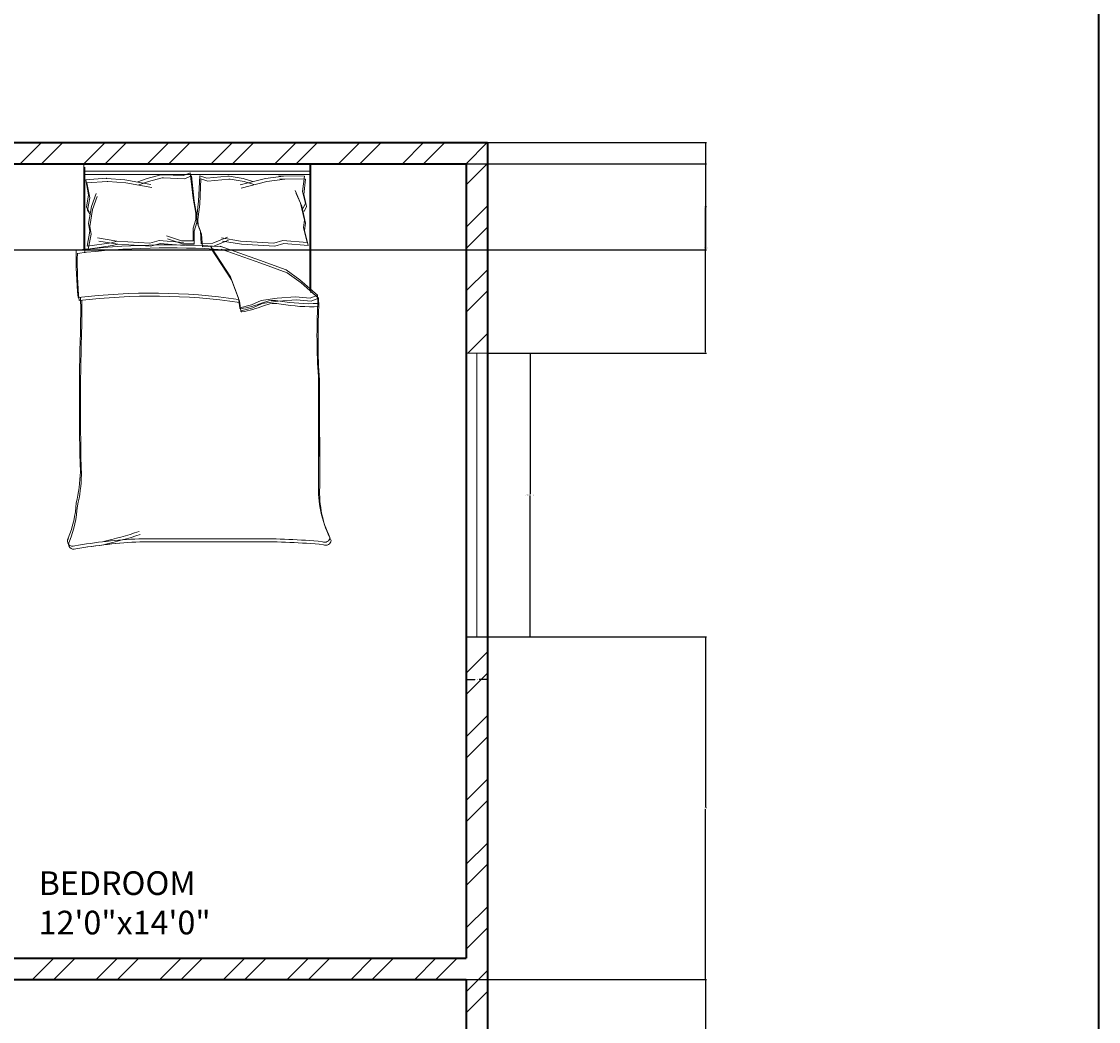
# Model space of a CAD drawing. Units: inches. Extents: x 392 to 1254, y 1207 to 2665.
# Tile 14 of 15: x 1026 to 1254, y 2043 to 2255. Entities that reach past the tile are written whole.
import ezdxf

# ---------------------------------------------------------------- set-up
doc = ezdxf.new("R2010")
doc.units = ezdxf.units.IN
for name, color, linetype, lineweight in [('A-ANNO-DIMS', 2, 'Continuous', 18), ('A-ANNO-TTLB', 7, 'Continuous', 35), ('A-AREA-IDEN', 7, 'Continuous', 18), ('A-FURN', 8, 'Continuous', 13), ('A-GLAZ', 4, 'Continuous', 18), ('A-WALL', 7, 'Continuous', 35), ('A-WALL-PATT', 252, 'Continuous', 13)]:
    doc.layers.add(name, color=color, linetype=linetype, lineweight=lineweight)
doc.styles.get("Standard").update_dxf_attribs({"font": 'arial.ttf'})
doc.dimstyles.get("Standard").update_dxf_attribs({"dimtxt": 0.18, "dimasz": 0.18, "dimexe": 0.18, "dimexo": 0.0625, "dimgap": 0.09, "dimtad": 0, "dimtih": 1, "dimtoh": 1, "dimdec": 4, "dimzin": 0, "dimdsep": 46, "dimtxsty": 'Standard', "dimcen": 0.09, "dimadec": 0, "dimazin": 0, "dimtfac": 1, "dimtdec": 4, "dimtofl": 0, "dimtmove": 0, "dimatfit": 3, "dimfxl": 1, "dimtolj": 1, "dimtzin": 0, "dimarcsym": 0})

# ---------------------------------------------------------------- blocks, each defined once
blk = doc.blocks.new('BED-DOUBLE')
for p, q in [((3.47, 63.33), (3.47, 81.44)), ((3.47, 79.91), (51.27, 79.91)), ((3.48, 63.33), (3.48, 81.44)), ((3.48, 79.91), (51.27, 79.91)), ((3.7, 62.69), (3.7, 80.8)), ((3.7, 62.69), (3.7, 80.8)), ((51.27, 81.44), (51.27, 54.83)), ((51.27, 81.44), (51.27, 54.83)), ((51.49, 81.44), (51.49, 80.8)), ((51.49, 80.8), (51.49, 54.19)), ((51.49, 80.8), (51.49, 54.19)), ((3.7, 79.27), (51.49, 79.27)), ((3.7, 79.27), (51.49, 79.27)), ((3.89, 78.13), (4.47, 74.95)), ((3.89, 78.13), (4.47, 74.95)), ((3.9, 78.1), (8.18, 78.43)), ((3.9, 78.1), (8.18, 78.43)), ((4.12, 77.49), (4.7, 74.31)), ((4.12, 77.49), (4.7, 74.31)), ((4.13, 77.47), (8.41, 77.79)), ((4.13, 77.47), (8.41, 77.79)), ((8.18, 78.43), (8.28, 78.42)), ((8.18, 78.43), (8.28, 78.42)), ((8.28, 78.42), (12.11, 78.13)), ((8.28, 78.42), (12.11, 78.13)), ((8.41, 77.79), (8.51, 77.78)), ((8.41, 77.79), (8.51, 77.78)), ((8.51, 77.78), (12.34, 77.49)), ((8.51, 77.78), (12.34, 77.49)), ((12.11, 78.13), (17.6, 77.11)), ((12.11, 78.13), (17.6, 77.11)), ((12.34, 77.49), (17.83, 76.48)), ((12.34, 77.49), (17.83, 76.48)), ((14.85, 77.69), (16.88, 78.42)), ((14.85, 77.69), (16.88, 78.42)), ((15.08, 77.05), (17.11, 77.78)), ((15.08, 77.05), (17.11, 77.78)), ((16.88, 78.42), (19.77, 79.14)), ((16.88, 78.42), (19.77, 79.14)), ((17.11, 77.78), (20, 78.5)), ((17.11, 77.78), (20, 78.5)), ((19.77, 79.14), (20.09, 79.14)), ((19.77, 79.14), (20.09, 79.14)), ((20, 78.5), (20.32, 78.5)), ((20, 78.5), (20.32, 78.5)), ((20.09, 79.14), (24.54, 78.99)), ((20.09, 79.14), (24.54, 78.99)), ((20.32, 78.5), (24.77, 78.35)), ((20.32, 78.5), (24.77, 78.35)), ((24.54, 78.99), (25.98, 79.57)), ((24.54, 78.99), (25.98, 79.57)), ((24.77, 78.35), (26.21, 78.93)), ((24.77, 78.35), (26.21, 78.93)), ((25.98, 79.57), (26.56, 74.22)), ((25.98, 79.57), (26.56, 74.22)), ((26.21, 78.93), (26.79, 73.58)), ((26.21, 78.93), (26.79, 73.58)), ((27.98, 78.95), (27.73, 73.58)), ((27.98, 78.95), (27.73, 73.58)), ((28.21, 78.31), (27.96, 72.94)), ((28.21, 78.31), (27.96, 72.94)), ((29.46, 78.46), (27.98, 78.95)), ((29.46, 78.46), (27.98, 78.95)), ((29.68, 77.82), (28.21, 78.31)), ((29.68, 77.82), (28.21, 78.31)), ((33.88, 78.89), (29.46, 78.46)), ((33.88, 78.89), (29.46, 78.46)), ((34.11, 78.25), (29.68, 77.82)), ((34.11, 78.25), (29.68, 77.82)), ((34.2, 78.91), (33.88, 78.89)), ((34.2, 78.91), (33.88, 78.89)), ((34.43, 78.27), (34.11, 78.25)), ((34.43, 78.27), (34.11, 78.25)), ((37.14, 78.36), (34.2, 78.91)), ((37.14, 78.36), (34.2, 78.91)), ((37.36, 77.73), (34.43, 78.27)), ((37.36, 77.73), (34.43, 78.27)), ((41.91, 78.37), (36.49, 77.02)), ((41.91, 78.37), (36.5, 77.02)), ((42.14, 77.73), (36.72, 76.38)), ((42.14, 77.73), (36.72, 76.38)), ((39.2, 77.77), (37.14, 78.36)), ((39.2, 77.77), (37.14, 78.36)), ((39.43, 77.13), (37.36, 77.73)), ((39.43, 77.13), (37.36, 77.73)), ((45.71, 78.9), (41.91, 78.37)), ((45.71, 78.9), (41.91, 78.37)), ((45.94, 78.26), (42.14, 77.73)), ((45.94, 78.26), (42.14, 77.73)), ((50.11, 78.89), (44.71, 78.98)), ((44.71, 78.98), (45.71, 78.9)), ((50.11, 78.89), (44.71, 78.98)), ((44.71, 78.98), (45.71, 78.9)), ((50.34, 78.25), (44.94, 78.34)), ((44.94, 78.34), (45.94, 78.26)), ((50.34, 78.25), (44.94, 78.34)), ((44.94, 78.34), (45.94, 78.26)), ((50.11, 78.89), (49.73, 75.67)), ((50.11, 78.89), (49.73, 75.67)), ((50.34, 78.25), (49.96, 75.04)), ((50.34, 78.25), (49.96, 75.04)), ((5.05, 72.49), (6.06, 75.23)), ((5.05, 72.49), (6.06, 75.23)), ((49.31, 73.19), (48.13, 75.86)), ((49.31, 73.19), (48.13, 75.86)), ((49.54, 72.55), (48.36, 75.22)), ((49.54, 72.55), (48.36, 75.22)), ((49.73, 75.67), (50.33, 73.1)), ((49.73, 75.67), (50.33, 73.1)), ((4.47, 74.95), (4.04, 72.34)), ((4.47, 74.95), (4.04, 72.34)), ((4.7, 74.31), (4.27, 71.7)), ((4.7, 74.31), (4.27, 71.7)), ((5.28, 71.85), (6.29, 74.6)), ((5.28, 71.85), (6.29, 74.6)), ((26.56, 74.22), (27.14, 71.04)), ((26.56, 74.22), (27.14, 71.04)), ((26.79, 73.58), (27.37, 70.4)), ((26.79, 73.58), (27.37, 70.4)), ((27.73, 73.58), (27.35, 70.36)), ((27.73, 73.58), (27.35, 70.36)), ((27.96, 72.94), (27.58, 69.73)), ((27.96, 72.94), (27.58, 69.73)), ((50.11, 69.61), (49.31, 73.19)), ((50.11, 69.61), (49.31, 73.19)), ((50.33, 73.1), (49.81, 72.06)), ((50.33, 73.1), (49.81, 72.06)), ((49.96, 75.04), (50.56, 72.47)), ((49.96, 75.04), (50.56, 72.47)), ((4.04, 72.34), (4.62, 71.33)), ((4.04, 72.34), (4.62, 71.33)), ((4.27, 71.7), (4.85, 70.69)), ((4.27, 71.7), (4.85, 70.69)), ((4.47, 68.87), (5.05, 72.49)), ((4.47, 68.87), (5.05, 72.49)), ((4.7, 68.23), (5.28, 71.85)), ((4.7, 68.23), (5.28, 71.85)), ((27.14, 71.04), (27.14, 69.74)), ((27.14, 71.04), (27.14, 69.74)), ((50.34, 68.97), (49.54, 72.55)), ((50.34, 68.97), (49.54, 72.55)), ((50.56, 72.47), (50.04, 71.42)), ((50.56, 72.47), (50.04, 71.42)), ((4.76, 67.28), (4.47, 68.87)), ((4.76, 67.28), (4.47, 68.87)), ((27.14, 69.74), (26.56, 67.86)), ((27.14, 69.74), (26.56, 67.86)), ((27.37, 69.1), (26.79, 67.22)), ((27.37, 69.1), (26.79, 67.22)), ((27.35, 70.36), (27.44, 69.07)), ((27.35, 70.36), (27.44, 69.07)), ((27.37, 70.4), (27.37, 69.1)), ((27.37, 70.4), (27.37, 69.1)), ((27.44, 69.07), (28.13, 67.23)), ((27.44, 69.07), (28.13, 67.23)), ((27.58, 69.73), (27.66, 68.43)), ((27.58, 69.73), (27.66, 68.43)), ((27.66, 68.43), (28.36, 66.59)), ((27.66, 68.43), (28.36, 66.59)), ((49.92, 68.01), (50.11, 69.61)), ((49.92, 68.01), (50.11, 69.61)), ((50.15, 67.37), (50.34, 68.97)), ((50.15, 67.37), (50.34, 68.97)), ((4.18, 64.1), (4.76, 67.28)), ((4.18, 64.1), (4.76, 67.28)), ((4.41, 63.46), (4.99, 66.64)), ((4.41, 63.46), (4.99, 66.64)), ((4.99, 66.64), (4.7, 68.23)), ((4.99, 66.64), (4.7, 68.23)), ((24.1, 65.18), (20.96, 66.27)), ((24.1, 65.18), (20.96, 66.27)), ((26.56, 67.86), (26.56, 65.18)), ((26.56, 67.86), (26.56, 65.18)), ((26.79, 67.22), (26.79, 64.54)), ((26.79, 67.22), (26.79, 64.54)), ((28.13, 67.23), (28.3, 64.55)), ((28.13, 67.23), (28.3, 64.55)), ((28.36, 66.59), (28.53, 63.91)), ((28.36, 66.59), (28.53, 63.91)), ((50.7, 64.87), (49.92, 68.01)), ((50.7, 64.87), (49.92, 68.01)), ((50.93, 64.23), (50.15, 67.37)), ((50.93, 64.23), (50.15, 67.37)), ((9.28, 64.82), (4.18, 64.1)), ((9.28, 64.82), (4.18, 64.1)), ((9.51, 64.19), (4.41, 63.46)), ((9.51, 64.19), (4.41, 63.46)), ((6.38, 65.81), (10.41, 65.15)), ((6.38, 65.81), (10.41, 65.15)), ((6.61, 65.17), (10.64, 64.51)), ((6.61, 65.17), (10.64, 64.51)), ((10.41, 65.15), (9.28, 64.82)), ((10.41, 65.15), (9.28, 64.82)), ((10.64, 64.51), (9.51, 64.19)), ((10.64, 64.51), (9.51, 64.19)), ((10.41, 65.15), (17.42, 64.72)), ((10.41, 65.15), (17.42, 64.72)), ((10.64, 64.51), (17.65, 64.08)), ((10.64, 64.51), (17.65, 64.08)), ((17.42, 64.72), (19.38, 65.27)), ((17.42, 64.72), (19.38, 65.27)), ((17.65, 64.08), (19.61, 64.63)), ((17.65, 64.08), (19.61, 64.63)), ((19.38, 65.27), (24.52, 64.87)), ((19.38, 65.27), (24.52, 64.87)), ((19.61, 64.63), (24.74, 64.23)), ((19.61, 64.63), (24.74, 64.23)), ((24.33, 64.54), (21.19, 65.63)), ((24.33, 64.54), (21.19, 65.63)), ((26.56, 65.18), (24.1, 65.18)), ((26.56, 65.18), (24.1, 65.18)), ((26.79, 64.54), (24.33, 64.54)), ((26.79, 64.54), (24.33, 64.54)), ((28.3, 64.55), (30.75, 64.7)), ((28.3, 64.55), (30.75, 64.7)), ((28.53, 63.91), (30.98, 64.06)), ((28.53, 63.91), (30.98, 64.06)), ((30.26, 64.06), (34.45, 57.57)), ((30.26, 64.06), (34.45, 57.57)), ((30.75, 64.7), (33.82, 65.99)), ((30.75, 64.7), (33.82, 65.99)), ((30.98, 64.06), (34.05, 65.35)), ((30.98, 64.06), (34.05, 65.35)), ((40.64, 61.13), (32.31, 64.06)), ((40.64, 61.13), (32.31, 64.06)), ((32.56, 65.81), (36.6, 65.15)), ((32.56, 65.81), (36.6, 65.15)), ((32.79, 65.17), (36.82, 64.51)), ((32.79, 65.17), (36.82, 64.51)), ((36.6, 65.15), (43.61, 64.72)), ((36.6, 65.15), (43.61, 64.72)), ((36.82, 64.51), (43.83, 64.08)), ((36.82, 64.51), (43.83, 64.08)), ((43.61, 64.72), (45.57, 65.27)), ((43.61, 64.72), (45.57, 65.27)), ((43.83, 64.08), (45.79, 64.63)), ((43.83, 64.08), (45.79, 64.63)), ((45.57, 65.27), (50.7, 64.87)), ((45.57, 65.27), (50.7, 64.87)), ((45.79, 64.63), (50.93, 64.23)), ((45.79, 64.63), (50.93, 64.23)), ((30.49, 63.42), (34.68, 56.93)), ((30.49, 63.42), (34.68, 56.93)), ((40.87, 60.49), (32.53, 63.42)), ((40.87, 60.49), (32.53, 63.42)), ((46.22, 59.11), (40.64, 61.13)), ((46.22, 59.11), (40.64, 61.13)), ((46.45, 58.47), (40.87, 60.49)), ((46.45, 58.47), (40.87, 60.49)), ((34.45, 57.57), (36.15, 53.08)), ((34.45, 57.57), (36.15, 53.08)), ((49.16, 56.95), (46.22, 59.11)), ((49.16, 56.95), (46.22, 59.11)), ((49.39, 56.31), (46.45, 58.47)), ((49.39, 56.31), (46.45, 58.47)), ((52.87, 53.7), (49.16, 56.95)), ((52.87, 53.7), (49.16, 56.95)), ((34.68, 56.93), (36.38, 52.44)), ((34.68, 56.93), (36.38, 52.44)), ((53.1, 53.06), (49.39, 56.31)), ((53.1, 53.06), (49.39, 56.31)), ((36.15, 53.08), (36.46, 51.07)), ((36.15, 53.08), (36.46, 51.07)), ((36.38, 52.44), (36.69, 50.43)), ((36.38, 52.44), (36.69, 50.43)), ((38.94, 51.68), (40.95, 52.61)), ((38.94, 51.68), (40.95, 52.61)), ((40.95, 52.61), (44.36, 53.08)), ((40.95, 52.61), (44.36, 53.08)), ((41.18, 51.97), (44.59, 52.44)), ((41.18, 51.97), (44.59, 52.44)), ((44.36, 53.08), (48.23, 53.39)), ((44.36, 53.08), (48.23, 53.39)), ((44.59, 52.44), (48.46, 52.75)), ((44.59, 52.44), (48.46, 52.75)), ((48.23, 53.39), (51.33, 53.08)), ((48.23, 53.39), (51.33, 53.08)), ((48.46, 52.75), (51.56, 52.44)), ((48.46, 52.75), (51.56, 52.44)), ((51.33, 53.08), (52.87, 53.7)), ((51.33, 53.08), (52.87, 53.7)), ((51.56, 52.44), (53.1, 53.06)), ((51.56, 52.44), (53.1, 53.06)), ((52.95, 51.95), (52.87, 53.7, 3.87)), ((52.95, 51.95), (52.87, 53.7, 3.87)), ((53.18, 51.31), (53.1, 53.06, 3.87)), ((53.18, 51.31), (53.1, 53.06, 3.87)), ((36.46, 51.07), (38.94, 51.68)), ((36.46, 51.07), (38.94, 51.68)), ((36.69, 50.43), (39.17, 51.05)), ((36.69, 50.43), (39.17, 51.05)), ((39.17, 51.05), (41.18, 51.97)), ((39.17, 51.05), (41.18, 51.97)), ((15.06, 2.2), (39.68, 2.2)), ((15.06, 2.2), (39.68, 2.2)), ((15.29, 1.56), (39.91, 1.56)), ((15.29, 1.56), (39.91, 1.56))]:
    blk.add_line(p, q)
for centre, radius, start, end in [((21.36, -100.61), 164.97, 86.0865, 96.7821), ((21.36, -100.61), 164.97, 86.0865, 96.7821), ((85.16, 61.35), 83.31, 178.7218, 185.604), ((85.16, 61.35), 83.31, 178.7218, 185.604), ((85.39, 60.71), 83.31, 178.7218, 185.604), ((85.39, 60.71), 83.31, 178.7218, 185.604), ((21.59, -101.25), 164.97, 86.0865, 96.7821), ((21.59, -101.25), 164.97, 86.0865, 96.7821), ((17.76, -74.87), 129.02, 81.7845, 96.9006), ((17.76, -74.87), 129.02, 81.7845, 96.9006), ((17.98, -75.51), 129.02, 81.7845, 96.9006), ((17.98, -75.51), 129.02, 81.7845, 96.9006), ((-167.31, 50.27), 170.11, 358.4762, 1.0082), ((-167.31, 50.27), 170.11, 358.4762, 1.0082), ((-167.08, 49.63), 170.11, 358.4762, 1.0082), ((-167.08, 49.63), 170.11, 358.4762, 1.0082), ((43.74, 46.38), 6.22, 78.6608, 113.7384), ((43.74, 46.38), 6.22, 78.6608, 113.7384), ((51.33, 88.1), 36.18, 259.8763, 272.5657), ((51.33, 88.1), 36.18, 259.8763, 272.5657), ((36.64, 51), 0.185, 160.2464, 271.1377), ((36.64, 51), 0.185, 160.2464, 271.1377), ((31.15, 79.96), 29.65, 280.6617, 289.8806), ((31.15, 79.96), 29.65, 280.6617, 289.8806), ((36.86, 50.36), 0.185, 160.2464, 271.1377), ((36.86, 50.36), 0.185, 160.2464, 271.1377), ((31.38, 79.32), 29.65, 280.6617, 289.8806), ((31.38, 79.32), 29.65, 280.6617, 289.8806), ((43.97, 45.74), 6.22, 78.6608, 113.7384), ((43.97, 45.74), 6.22, 78.6608, 113.7384), ((51.56, 87.46), 36.18, 259.8763, 272.5657), ((51.56, 87.46), 36.18, 259.8763, 272.5657), ((182.27, 45.13), 129.5, 176.9791, 183.8365), ((182.27, 45.13), 129.5, 176.9791, 183.8365), ((182.49, 44.49), 129.5, 176.9791, 183.8365), ((182.49, 44.49), 129.5, 176.9791, 183.8365), ((484.82, 30.83), 482.31, 178.2277, 181.7185), ((484.82, 30.83), 482.31, 178.2277, 181.7185), ((485.05, 30.19), 482.31, 178.2277, 181.7185), ((485.05, 30.19), 482.31, 178.2277, 181.7185), ((-4508.74, 13.62), 4561.86, 0.00217, 0.28689), ((-4508.74, 13.62), 4561.86, 0.00217, 0.28689), ((-4508.51, 12.98), 4561.86, 0.00217, 0.28689), ((-4508.52, 12.98), 4561.86, 0.00217, 0.28689), ((-26.9, 16.93), 29.63, 346.0648, 358.9113), ((-26.9, 16.93), 29.63, 346.0648, 358.9113), ((-26.67, 16.29), 29.63, 346.0648, 358.9113), ((-26.67, 16.29), 29.63, 346.0648, 358.9113), ((76.16, 12.78), 23.07, 177.4714, 206.4681), ((76.16, 12.78), 23.07, 177.4714, 206.4681), ((76.39, 12.14), 23.07, 177.4714, 206.4681), ((76.39, 12.14), 23.07, 177.4714, 206.4681), ((-21.66, 11.17), 23.56, 337.9751, 356.652), ((-21.66, 11.17), 23.56, 337.9751, 356.652), ((-21.43, 10.53), 23.56, 337.9751, 356.652), ((-21.43, 10.53), 23.56, 337.9751, 356.652), ((1.09, 1.72), 1.09, 146.1736, 293.4781), ((1.09, 1.72), 1.09, 146.1736, 293.4781), ((-17.22, 105.15), 106.46, 283.3832, 287.7053), ((-17.22, 105.15), 106.46, 283.3832, 287.7053), ((-16.99, 104.52), 106.46, 283.3832, 287.7053), ((-16.99, 104.52), 106.46, 283.3832, 287.7053), ((54.41, 2.57), 1.1, 242.6588, 356.02), ((54.41, 2.57), 1.1, 242.6588, 356.02), ((1.32, 1.09), 1.09, 146.1736, 293.4781), ((1.32, 1.09), 1.09, 146.1736, 293.4781), ((21.43, -119.39), 121.76, 92.9958, 99.4091), ((21.43, -119.39), 121.76, 92.9958, 99.4091), ((21.66, -120.03), 121.76, 92.9958, 99.4091), ((21.65, -120.03), 121.76, 92.9958, 99.4091), ((41.15, -130.83), 133.04, 84.4998, 90.6351), ((41.15, -130.83), 133.04, 84.4998, 90.6351), ((41.38, -131.47), 133.04, 84.4998, 90.6351), ((41.38, -131.47), 133.04, 84.4998, 90.6351), ((54.64, 1.93), 1.1, 242.6588, 356.02), ((54.64, 1.93), 1.1, 242.6588, 356.02)]:
    blk.add_arc(centre, radius, start, end)
blk = doc.blocks.new('WIN-60-A')
for p, q in [((0, 60), (4.5, 60)), ((4.5, 60), (2.25, 60)), ((2.25, 60), (2.25, 0)), ((2.25, 0), (0, 0)), ((0, 0), (4.5, 0))]:
    blk.add_line(p, q)
blk = doc.blocks.new('*D11')
at = {"layer": 'A-ANNO-DIMS', "color": 0, "lineweight": -2, "transparency": 16777216}
for p, q in [((1124.84, 2184.76), (1133.96, 2184.76)), ((1133.78, 2184.58), (1133.78, 2154.94)), ((1133.78, 2124.94), (1133.78, 2154.58)), ((1124.84, 2124.76), (1133.96, 2124.76))]:
    blk.add_line(p, q, dxfattribs=at)
at = {"layer": 'A-ANNO-DIMS', "color": 0, "transparency": 16777216}
for points in [[(1133.75, 2184.58), (1133.81, 2184.58), (1133.78, 2184.76)], [(1133.75, 2124.94), (1133.81, 2124.94), (1133.78, 2124.76)]]:
    blk.add_solid(points, dxfattribs=at)
at = {"layer": 'Defpoints', "color": 0, "transparency": 16777216}
for p in [(1124.78, 2184.76), (1124.78, 2124.76), (1133.78, 2124.76)]:
    blk.add_point(p, dxfattribs=at)
at = {"layer": 'A-ANNO-DIMS', "color": 0, "transparency": 16777216, "insert": (1133.78, 2154.76), "char_height": 0.18, "attachment_point": 5}
blk.add_mtext('\\A1;WINDOW A 60 TYP.', dxfattribs=at)
blk = doc.blocks.new('*D12')
at = {"layer": 'A-ANNO-DIMS', "color": 0, "lineweight": -2, "transparency": 16777216}
for p, q in [((1120.28, 2124.7), (1120.28, 2115.58)), ((1124.78, 2124.7), (1124.78, 2115.58)), ((1120.46, 2115.76), (1122.07, 2115.76)), ((1124.6, 2115.76), (1122.99, 2115.76))]:
    blk.add_line(p, q, dxfattribs=at)
at = {"layer": 'A-ANNO-DIMS', "color": 0, "transparency": 16777216}
for points in [[(1120.46, 2115.79), (1120.46, 2115.73), (1120.28, 2115.76)], [(1124.6, 2115.79), (1124.6, 2115.73), (1124.78, 2115.76)]]:
    blk.add_solid(points, dxfattribs=at)
at = {"layer": 'Defpoints', "color": 0, "transparency": 16777216}
for p in [(1120.28, 2124.76), (1124.78, 2124.76), (1120.28, 2115.76)]:
    blk.add_point(p, dxfattribs=at)
at = {"layer": 'A-ANNO-DIMS', "color": 0, "transparency": 16777216, "insert": (1122.53, 2115.76), "char_height": 0.18, "attachment_point": 5}
blk.add_mtext('\\A1;5 TYP.', dxfattribs=at)
blk = doc.blocks.new('*D34')
at = {"layer": 'A-ANNO-DIMS', "color": 0, "lineweight": -2, "transparency": 16777216}
for p, q in [((1120.34, 2124.76), (1171.06, 2124.76)), ((1170.88, 2124.58), (1170.88, 2088.71)), ((1170.88, 2052.48), (1170.88, 2088.35)), ((1120.34, 2052.3), (1171.06, 2052.3))]:
    blk.add_line(p, q, dxfattribs=at)
at = {"layer": 'A-ANNO-DIMS', "color": 0, "transparency": 16777216}
for points in [[(1170.85, 2124.58), (1170.91, 2124.58), (1170.88, 2124.76)], [(1170.85, 2052.48), (1170.91, 2052.48), (1170.88, 2052.3)]]:
    blk.add_solid(points, dxfattribs=at)
at = {"layer": 'Defpoints', "color": 0, "transparency": 16777216}
for p in [(1120.28, 2124.76), (1170.88, 2124.76), (1120.28, 2052.3)]:
    blk.add_point(p, dxfattribs=at)
at = {"layer": 'A-ANNO-DIMS', "color": 0, "transparency": 16777216, "insert": (1170.88, 2088.53), "char_height": 0.18, "attachment_point": 5}
blk.add_mtext('\\A1;72.47', dxfattribs=at)
blk = doc.blocks.new('*D39')
at = {"layer": 'A-ANNO-DIMS', "color": 0, "lineweight": -2, "transparency": 16777216}
for p, q in [((1124.84, 2229.3), (1171.06, 2229.3)), ((1170.88, 2229.12), (1170.88, 2207.21)), ((1170.88, 2184.94), (1170.88, 2206.85)), ((1124.84, 2184.76), (1171.06, 2184.76))]:
    blk.add_line(p, q, dxfattribs=at)
at = {"layer": 'A-ANNO-DIMS', "color": 0, "transparency": 16777216}
for points in [[(1170.85, 2229.12), (1170.91, 2229.12), (1170.88, 2229.3)], [(1170.85, 2184.94), (1170.91, 2184.94), (1170.88, 2184.76)]]:
    blk.add_solid(points, dxfattribs=at)
at = {"layer": 'Defpoints', "color": 0, "transparency": 16777216}
for p in [(1124.78, 2229.3), (1124.78, 2184.76), (1170.88, 2184.76)]:
    blk.add_point(p, dxfattribs=at)
at = {"layer": 'A-ANNO-DIMS', "color": 0, "transparency": 16777216, "insert": (1170.88, 2207.03), "char_height": 0.18, "attachment_point": 5}
blk.add_mtext('\\A1;44.535', dxfattribs=at)
blk = doc.blocks.new('*D40')
at = {"layer": 'A-ANNO-DIMS', "color": 0, "lineweight": -2, "transparency": 16777216}
for p, q in [((1120.34, 2052.3), (1171.06, 2052.3)), ((1170.88, 2052.12), (1170.88, 2022.56)), ((1170.88, 1992.64), (1170.88, 2022.19)), ((1120.34, 1992.46), (1171.06, 1992.46))]:
    blk.add_line(p, q, dxfattribs=at)
at = {"layer": 'A-ANNO-DIMS', "color": 0, "transparency": 16777216}
for points in [[(1170.85, 2052.12), (1170.91, 2052.12), (1170.88, 2052.3)], [(1170.85, 1992.64), (1170.91, 1992.64), (1170.88, 1992.46)]]:
    blk.add_solid(points, dxfattribs=at)
at = {"layer": 'Defpoints', "color": 0, "transparency": 16777216}
for p in [(1120.28, 2052.3), (1120.28, 1992.46), (1170.88, 1992.46)]:
    blk.add_point(p, dxfattribs=at)
at = {"layer": 'A-ANNO-DIMS', "color": 0, "transparency": 16777216, "insert": (1170.88, 2022.38), "char_height": 0.18, "attachment_point": 5}
blk.add_mtext('\\A1;59.84', dxfattribs=at)
blk = doc.blocks.new('*D79')
at = {"layer": 'A-ANNO-DIMS', "color": 0, "lineweight": -2, "transparency": 16777216}
for p, q in [((830.84, 2224.8), (1171.06, 2224.8)), ((1170.88, 2224.62), (1170.88, 2215.87)), ((1170.88, 2206.76), (1170.88, 2215.5)), ((830.84, 2206.58), (1171.06, 2206.58))]:
    blk.add_line(p, q, dxfattribs=at)
at = {"layer": 'A-ANNO-DIMS', "color": 0, "transparency": 16777216}
for points in [[(1170.85, 2224.62), (1170.91, 2224.62), (1170.88, 2224.8)], [(1170.85, 2206.76), (1170.91, 2206.76), (1170.88, 2206.58)]]:
    blk.add_solid(points, dxfattribs=at)
at = {"layer": 'Defpoints', "color": 0, "transparency": 16777216}
for p in [(830.78, 2224.8), (1170.88, 2224.8), (830.78, 2206.58)]:
    blk.add_point(p, dxfattribs=at)
at = {"layer": 'A-ANNO-DIMS', "color": 0, "transparency": 16777216, "insert": (1170.88, 2215.69), "char_height": 0.18, "attachment_point": 5}
blk.add_mtext('\\A1;18.22', dxfattribs=at)

msp = doc.modelspace()

# ---------------------------------------------------------------- hatches: boundary and pattern name
at = {"layer": 'A-WALL-PATT'}
h = msp.add_hatch(dxfattribs=at)
h.set_pattern_fill('ANSI32', color=256)
h.paths.add_polyline_path([(579.5309, 2227.0453), (579.5309, 2229.2953), (541.2807, 2229.2953), (541.2807, 2182.3091), (545.7807, 2182.3091), (545.7807, 2224.7953), (579.5309, 2224.7953)])
h.paths.add_polyline_path([(655.4442, 2229.2953), (627.5309, 2229.2953), (627.5309, 2224.7953), (655.4442, 2224.7953), (655.4442, 2227.0453)])
h.paths.add_polyline_path([(703.0758, 2229.2953), (678.5257, 2229.2953), (678.5257, 2227.0453), (678.5257, 2224.7953), (689.7807, 2224.7953), (689.7807, 2158.6973), (694.2807, 2158.6973), (694.2807, 2224.7953), (703.0758, 2224.7953)])
h.paths.add_polyline_path([(768.5767, 2229.2953), (727.0758, 2229.2953), (727.0758, 2224.7953), (742.2807, 2224.7953), (742.2807, 2128.7953), (694.2807, 2128.7953), (694.2807, 2134.0554), (689.7807, 2134.0554), (689.7807, 2090.2854), (694.2807, 2090.2854), (694.2807, 2124.2953), (742.2807, 2124.2953), (742.2807, 2052.2953), (795.2124, 2052.2953), (795.2124, 2054.5453), (795.2124, 2056.7953), (746.7807, 2056.7953), (746.7807, 2224.7953), (768.5767, 2224.7953)])
h.paths.add_polyline_path([(867.5089, 2229.2953), (804.5767, 2229.2953), (804.5767, 2224.7953), (830.7807, 2224.7953), (830.7807, 2056.7953), (826.9066, 2056.7953), (826.9066, 2052.2953), (830.7807, 2052.2953), (830.7807, 1886.6777, -0.01766664), (830.8602, 1884.2953), (835.0818, 1884.2953, -0.04411348), (835.2807, 1889.9369), (835.2807, 2052.2953), (839.418, 2052.2953), (839.418, 2056.7953), (835.2807, 2056.7953), (835.2807, 2224.7953), (867.5089, 2224.7953)])
h.paths.add_polyline_path([(939.8604, 2229.2953), (903.5089, 2229.2953), (903.5089, 2227.0453), (903.5089, 2224.7953), (919.2807, 2224.7953), (919.2807, 2056.7953), (870.6499, 2056.7953), (870.6499, 2052.2953), (923.7807, 2052.2953), (923.7807, 2124.2953), (971.7807, 2124.2953), (971.7807, 2089.7112), (974.0307, 2089.7112), (976.2807, 2089.7112), (976.2807, 2133.56), (974.0307, 2133.56), (971.7807, 2133.56), (971.7807, 2128.7953), (923.7807, 2128.7953), (923.7807, 2224.7953), (939.8604, 2224.7953)])
h.paths.add_polyline_path([(1124.7807, 2229.2953), (1009.403, 2229.2953), (1009.403, 2224.7953), (1120.2807, 2224.7953), (1120.2807, 2184.7605), (1124.7807, 2184.7605)])
h.paths.add_polyline_path([(1124.7807, 2124.7605), (1120.2807, 2124.7605), (1120.2807, 2056.7953), (976.2807, 2056.7953), (976.2807, 2061.471), (971.7807, 2061.471), (971.7807, 2047.7483), (974.0307, 2047.7483), (976.2807, 2047.7483), (976.2807, 2052.2953), (1120.2807, 2052.2953), (1120.2807, 1992.457), (1124.7807, 1992.457)])
h.paths.add_polyline_path([(1124.7807, 1932.457), (1122.5307, 1932.457), (1120.2807, 1932.457), (1120.2807, 1884.2953), (976.2807, 1884.2953), (976.2807, 2019.9536), (971.7807, 2019.9536), (971.7807, 1884.2953), (869.0911, 1884.2953), (869.0911, 1879.7953), (971.7807, 1879.7953), (1013.7807, 1879.7953), (1013.7807, 1831.7953), (971.7807, 1831.7953), (971.7807, 1822.3831), (974.0307, 1822.3831), (976.2807, 1822.3831), (976.2807, 1827.2953), (1013.7807, 1827.2953), (1025.6191, 1827.2953), (1025.6191, 1829.5453), (1025.6191, 1831.7953), (1018.2807, 1831.7953), (1018.2807, 1879.7953), (1120.2807, 1879.7953), (1120.2807, 1866.9192), (1124.7807, 1866.9192)])
h.paths.add_polyline_path([(1124.7807, 1842.9192), (1122.5307, 1842.9192), (1120.2807, 1842.9192), (1120.2807, 1831.7953), (1050.2021, 1831.7953), (1050.2021, 1827.2953), (1120.2807, 1827.2953), (1120.2807, 1781.4559), (1124.7807, 1781.4559)])
h.paths.add_polyline_path([(976.2807, 1790.8718), (971.7807, 1790.8718), (971.7807, 1648.3339), (976.2807, 1648.3339), (976.2807, 1654.7953), (1120.2807, 1654.7953), (1120.2807, 1626.3807), (1124.7807, 1626.3807), (1124.7807, 1721.4559), (1120.2807, 1721.4559), (1120.2807, 1659.2953), (976.2807, 1659.2953)])
h.paths.add_polyline_path([(1124.7807, 1566.3807), (1120.2807, 1566.3807), (1120.2807, 1486.7953), (1101.07, 1486.7953), (1101.07, 1482.2953), (1124.7807, 1482.2953)])
h.paths.add_polyline_path([(1041.07, 1484.5453), (1041.07, 1486.7953), (1006.2807, 1486.7953), (1006.2807, 1484.5453), (1006.2807, 1482.2953), (1041.07, 1482.2953)])
h.paths.add_polyline_path([(976.2807, 1617.5497), (974.0307, 1617.5497), (971.7807, 1617.5497), (971.7807, 1599.2953), (965.8041, 1599.2953), (965.8041, 1594.7953), (971.7807, 1594.7953), (971.7807, 1486.7953), (954.1249, 1486.7953), (954.1249, 1482.2953), (981.5717, 1482.2953), (981.5717, 1484.5453), (981.5717, 1486.7953), (976.2807, 1486.7953)])
h.paths.add_polyline_path([(930.1249, 1486.7953), (887.7807, 1486.7953), (887.7807, 1594.7953), (941.9141, 1594.7953), (941.9141, 1597.0453), (941.9141, 1599.2953), (887.7807, 1599.2953), (887.7807, 1659.2953), (863.5916, 1659.2953), (863.5916, 1654.7953), (883.2807, 1654.7953), (883.2807, 1438.7953), (782.7807, 1438.7953), (782.7807, 1486.7953), (782.7807, 1654.7953), (800.1309, 1654.7953), (800.1309, 1657.0453), (800.1309, 1659.2953), (778.2807, 1659.2953), (778.2807, 1599.2953), (721.7333, 1599.2953), (721.7333, 1597.0453), (721.7333, 1594.7953), (778.2807, 1594.7953), (778.2807, 1486.7953), (729.598, 1486.7953), (729.598, 1482.2953), (753.2885, 1482.2953), (753.2885, 1410.2953), (922.9852, 1410.2953), (922.9852, 1482.2953), (930.1249, 1482.2953)])
h.paths.add_polyline_path([(918.4852, 1482.2953), (918.4852, 1414.7953), (757.7885, 1414.7953), (757.7885, 1482.2953), (778.2807, 1482.2953), (778.2807, 1434.2953), (782.7807, 1434.2953), (887.7807, 1434.2953), (887.7807, 1438.7953), (887.7807, 1482.2953)], flags=16)
h.paths.add_polyline_path([(694.2807, 1594.7953), (700.4169, 1594.7953), (700.4169, 1597.0453), (700.4169, 1599.2953), (694.2807, 1599.2953), (694.2807, 1617.7503), (692.0307, 1617.7503), (689.7807, 1617.7503), (689.7807, 1486.7953), (682.7672, 1486.7953), (682.7672, 1482.2953), (705.598, 1482.2953), (705.598, 1484.5453), (705.598, 1486.7953), (694.2807, 1486.7953)])
h.paths.add_polyline_path([(545.7807, 1654.7953), (689.7807, 1654.7953), (689.7807, 1649.7691), (694.2807, 1649.7691), (694.2807, 1789.3981), (692.0307, 1789.3981), (689.7807, 1789.3981), (689.7807, 1659.2953), (545.7807, 1659.2953), (545.7807, 1714.4681), (543.5307, 1714.4681), (541.2807, 1714.4681), (541.2807, 1482.2953), (567.0628, 1482.2953), (567.0628, 1484.5453), (567.0628, 1486.7953), (545.7807, 1486.7953)])
h.paths.add_polyline_path([(545.7807, 1827.2953), (620.2247, 1827.2953), (620.2247, 1829.5453), (620.2247, 1831.7953), (545.7807, 1831.7953), (545.7807, 1846.8518), (541.2807, 1846.8518), (541.2807, 1774.4681), (545.7807, 1774.4681)])
h.paths.add_polyline_path([(797.0944, 1884.2953), (694.2807, 1884.2953), (694.2807, 2019.0288), (692.0307, 2019.0288), (689.7807, 2019.0288), (689.7807, 1884.2953), (545.7807, 1884.2953), (545.7807, 1951.8244), (541.2807, 1951.8244), (541.2807, 1870.8518), (543.5307, 1870.8518), (545.7807, 1870.8518), (545.7807, 1879.7953), (647.7807, 1879.7953), (647.7807, 1831.7953), (642.6413, 1831.7953), (642.6413, 1827.2953), (652.2807, 1827.2953), (689.7807, 1827.2953), (689.7807, 1821.0531), (694.2807, 1821.0531), (694.2807, 1831.7953), (652.2807, 1831.7953), (652.2807, 1879.7953), (797.0944, 1879.7953), (797.0944, 1882.0453)])
h.paths.add_polyline_path([(545.7807, 2122.3091), (541.2807, 2122.3091), (541.2807, 2011.8244), (543.5307, 2011.8244), (545.7807, 2011.8244), (545.7807, 2052.2953), (689.7807, 2052.2953), (689.7807, 2048.2048), (694.2807, 2048.2048), (694.2807, 2061.3129), (692.0307, 2061.3129), (689.7807, 2061.3129), (689.7807, 2056.7953), (545.7807, 2056.7953)])

# ---------------------------------------------------------------- linework, layer by layer
at = {"layer": 'A-ANNO-TTLB'}
msp.add_lwpolyline([(391.939, 2664.8979), (1253.97, 2664.8979), (1253.97, 1207.2611), (391.939, 1207.2611)], close=True, dxfattribs=at)
at = {"layer": 'A-WALL'}
for p, q in [((1007.5313, 2229.2953), (1124.7807, 2229.2953)), ((1124.7807, 2229.2953), (1124.7807, 1482.2953)), ((1009.403, 2224.7953), (1120.2807, 2224.7953)), ((1120.2807, 2224.7953), (1120.2807, 2056.7953)), ((976.2807, 2056.7953), (1120.2807, 2056.7953)), ((976.2807, 2052.2953), (1120.2807, 2052.2953)), ((1120.2807, 2052.2953), (1120.2807, 1884.2953))]:
    msp.add_line(p, q, dxfattribs=at)

# ---------------------------------------------------------------- block references
at = {"layer": 'A-FURN'}
msp.add_blockref('BED-DOUBLE', (1035.9344, 2143.3004), dxfattribs=at)
at = {"layer": 'A-GLAZ', "rotation": 180}
msp.add_blockref('WIN-60-A', (1124.7804, 2184.7606), dxfattribs=at)

# ---------------------------------------------------------------- texts
at = {"layer": 'A-AREA-IDEN', "insert": (1029.8415, 2075.1907), "char_height": 5, "attachment_point": 1}
msp.add_mtext_dynamic_manual_height_columns('BEDROOM\\P12\'0"x14\'0"', width=142.55623, gutter_width=12.5, heights=[0], dxfattribs=at)

# ---------------------------------------------------------------- dimensions: what is measured, and where the dimension line sits
at = {"layer": 'A-ANNO-DIMS'}
for base, p1, p2, override, picture, middle in [((1170.8807, 2184.7605), (1124.7807, 2229.2953), (1124.7807, 2184.7605), {"dimdec": 3, "dimlfac": 1, "dimrnd": 0, "dimzin": 0, "dimdsep": 46, "dimlunit": 2}, '*D39', (1170.8807, 2207.0279)), ((1170.8807, 2224.7953), (830.7807, 2206.5771), (830.7807, 2224.7953), {"dimdec": 2, "dimlfac": 1, "dimrnd": 0, "dimzin": 0, "dimdsep": 46, "dimlunit": 2}, '*D79', (1170.8807, 2215.6862)), ((1170.8807, 2124.7605), (1120.2807, 2052.2953), (1120.2807, 2124.7605), {"dimdec": 2, "dimlfac": 1, "dimrnd": 0, "dimzin": 0, "dimdsep": 46, "dimlunit": 2}, '*D34', (1170.8807, 2088.5279)), ((1170.8807, 1992.457), (1120.2807, 2052.2953), (1120.2807, 1992.457), {"dimdec": 2, "dimlfac": 1, "dimrnd": 0, "dimzin": 0, "dimdsep": 46, "dimlunit": 2}, '*D40', (1170.8807, 2022.3762))]:
    dim = msp.add_linear_dim(base=base, p1=p1, p2=p2, angle=90, dimstyle='Standard', override=override, dxfattribs=at)
    dim.commit()
    dim.dimension.update_dxf_attribs({"geometry": picture, "text_midpoint": middle})
for base, p1, p2, angle, text, picture, middle in [((1133.7807, 2124.7605), (1124.7807, 2184.7605), (1124.7807, 2124.7605), 270, 'WINDOW A <> TYP.', '*D11', (1133.7807, 2154.7605)), ((1120.2807091188, 2115.760528833), (1124.7807091188, 2124.760528833), (1120.2807091188, 2124.760528833), 180, '<> TYP.', '*D12', (1122.5307091188, 2115.760528833))]:
    dim = msp.add_linear_dim(base=base, p1=p1, p2=p2, angle=angle, text=text, dimstyle='Standard', override={"dimdec": 0, "dimlfac": 1, "dimrnd": 0, "dimzin": 0, "dimdsep": 46, "dimlunit": 2}, dxfattribs=at)
    dim.commit()
    dim.dimension.update_dxf_attribs({"geometry": picture, "text_midpoint": middle})

doc.saveas('drawing.dxf')
